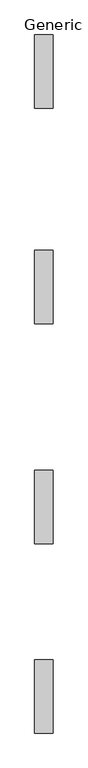
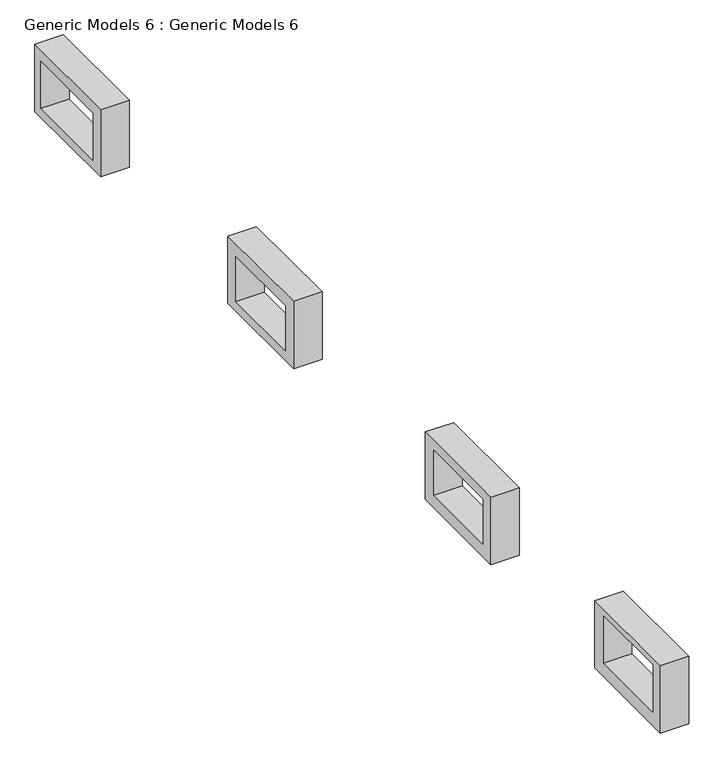
"""IFC4 building model written with IfcOpenShell, lengths in millimetres: proxy geometry, Generic Models 6 : Generic Models 6."""

from ifc_helpers import new_model, si_unit, frame, origin, place, context, project, spatial, polyline, outline, extrude, source, transform, mapped, element, save


def generic_models_6_generic_models_6_aab6ac76(model_context):
    return source(origin(), model_context, "Body", "SweptSolid", [
        extrude(outline(polyline([(5196.228718, 1209.0071283), (6415.428718, 1209.0071283), (6415.428718, 447.0071283), (5196.228718, 447.0071283), (5196.228718, 1209.0071283)]), holes=[polyline([(5341.7158406, 1082.1435071), (5341.7158406, 548.7435071), (6306.9158406, 548.7435071), (6306.9158406, 1082.1435071), (5341.7158406, 1082.1435071)])]), frame((-6675.0589614, 0.0, 0.0), z_axis=(1.0, 0.0, 0.0), x_axis=(0.0, 1.0, 0.0)), (0.0, 0.0, 1.0), 304.8),
        extrude(outline(polyline([(1614.828718, 1209.0071283), (2834.028718, 1209.0071283), (2834.028718, 447.0071283), (1614.828718, 447.0071283), (1614.828718, 1209.0071283)]), holes=[polyline([(1773.6692663, 1063.8916149), (1773.6692663, 555.8916149), (2688.0692663, 555.8916149), (2688.0692663, 1063.8916149), (1773.6692663, 1063.8916149)])]), frame((-6675.0589614, 0.0, 0.0), z_axis=(1.0, 0.0, 0.0), x_axis=(0.0, 1.0, 0.0)), (0.0, 0.0, 1.0), 304.8),
        extrude(outline(polyline([(-2042.771282, 1209.0071283), (-823.571282, 1209.0071283), (-823.571282, 447.0071283), (-2042.771282, 447.0071283), (-2042.771282, 1209.0071283)]), holes=[polyline([(-1896.4561758, 1095.0490461), (-1896.4561758, 587.0490461), (-982.0561758, 587.0490461), (-982.0561758, 1095.0490461), (-1896.4561758, 1095.0490461)])]), frame((-6675.0589614, 0.0, 0.0), z_axis=(1.0, 0.0, 0.0), x_axis=(0.0, 1.0, 0.0)), (0.0, 0.0, 1.0), 304.8),
        extrude(outline(polyline([(-5191.4109248, 1209.0071283), (-3972.2109248, 1209.0071283), (-3972.2109248, 447.0071283), (-5191.4109248, 447.0071283), (-5191.4109248, 1209.0071283)]), holes=[polyline([(-5049.5461038, 1132.2668128), (-5049.5461038, 598.8668128), (-4135.1461038, 598.8668128), (-4135.1461038, 1132.2668128), (-5049.5461038, 1132.2668128)])]), frame((-6675.0589614, 0.0, 0.0), z_axis=(1.0, 0.0, 0.0), x_axis=(0.0, 1.0, 0.0)), (0.0, 0.0, 1.0), 304.8),
    ])


if __name__ == "__main__":
    model = new_model("IFC4")
    model_context = context("Model", 3, world=origin())
    ifc_project = project(units=[si_unit("LENGTHUNIT", "METRE", prefix="MILLI")], contexts=[model_context])
    site = spatial("IfcSite", under=ifc_project)
    building = spatial("IfcBuilding", under=site)
    placement = place(None, origin())
    generic_models_6_generic_models_6_shape = generic_models_6_generic_models_6_aab6ac76(model_context)
    element("IfcBuildingElementProxy", 1, Name="Generic Models 6 : Generic Models 6", ObjectType="Generic Models 6 : Generic Models 6", at=placement, inside=building, context=model_context, shape_type="MappedRepresentation", body=[
        mapped(generic_models_6_generic_models_6_shape, transform((0.0, 0.0, 0.0), x_axis=(1.0, 0.0, 0.0), y_axis=(0.0, 1.0, 0.0), z_axis=(0.0, 0.0, 1.0))),
    ])
    save(model, "model.ifc")

# Revit data of these elements
# Element 1 (IfcBuildingElementProxy, "Generic Models 6 : Generic Models 6")
#   Materials on its faces: "Parking Stripe"
# Materials
#   "Parking Stripe": class "Paint", colour RGB 250 250 91, transparency 0, Cost = 0
